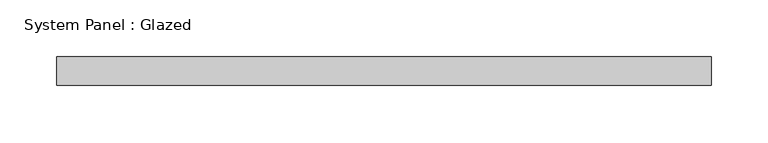
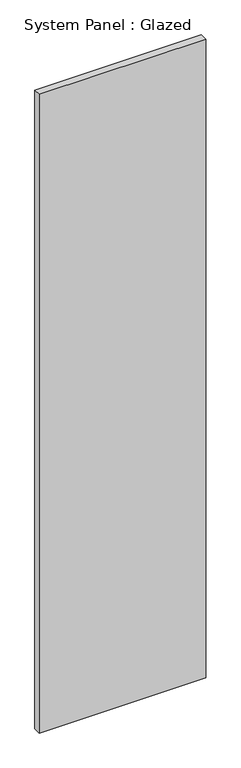
"""IFC4 building model written with IfcOpenShell, lengths in millimetres: plate geometry, System Panel : Glazed."""

from ifc_helpers import new_model, si_unit, origin, origin_with_axes, place, context, project, spatial, polyline, outline, extrude, source, transform, mapped, element, save


def system_panel_glazed_bb2333a0(model_context):
    return source(origin(), model_context, "Body", "SweptSolid", [
        extrude(outline(polyline([(288.925, -44.45), (-288.925, -44.45), (-288.925, -19.05), (288.925, -19.05), (288.925, -44.45)])), origin_with_axes(), (0.0, 0.0, 1.0), 2343.15),
    ])


if __name__ == "__main__":
    model = new_model("IFC4")
    model_context = context("Model", 3, world=origin())
    ifc_project = project(units=[si_unit("LENGTHUNIT", "METRE", prefix="MILLI")], contexts=[model_context])
    site = spatial("IfcSite", under=ifc_project)
    building = spatial("IfcBuilding", under=site)
    placement = place(None, origin())
    system_panel_glazed_shape = system_panel_glazed_bb2333a0(model_context)
    element("IfcPlate", 1, ObjectType="System Panel : Glazed", at=placement, inside=building, context=model_context, shape_type="MappedRepresentation", body=[
        mapped(system_panel_glazed_shape, transform((0.0, 0.0, 0.0), x_axis=(1.0, 0.0, 0.0), y_axis=(0.0, 1.0, 0.0), z_axis=(0.0, 0.0, 1.0))),
    ])
    save(model, "model.ifc")

# Revit data of these elements
# Type "System Panel : Glazed"
#   Construction Type Id = "GSP4R"
#   Analytic Construction = "1/8 in Pilkington single glazing"
#   Visual Light Transmittance = 0.9
#   Solar Heat Gain Coefficient = 0.86
#   Heat Transfer Coefficient (U) = 1.18115 BTU/(h·ft²·°F)
# Element 1 (IfcPlate, "System Panel : Glazed")
#   Materials on its faces: "Glass"
# Materials
#   "Glass": class "Glass", colour RGB 0 128 192, transparency 0.75, Description = "Soda Lime Glass", Cost = 0
